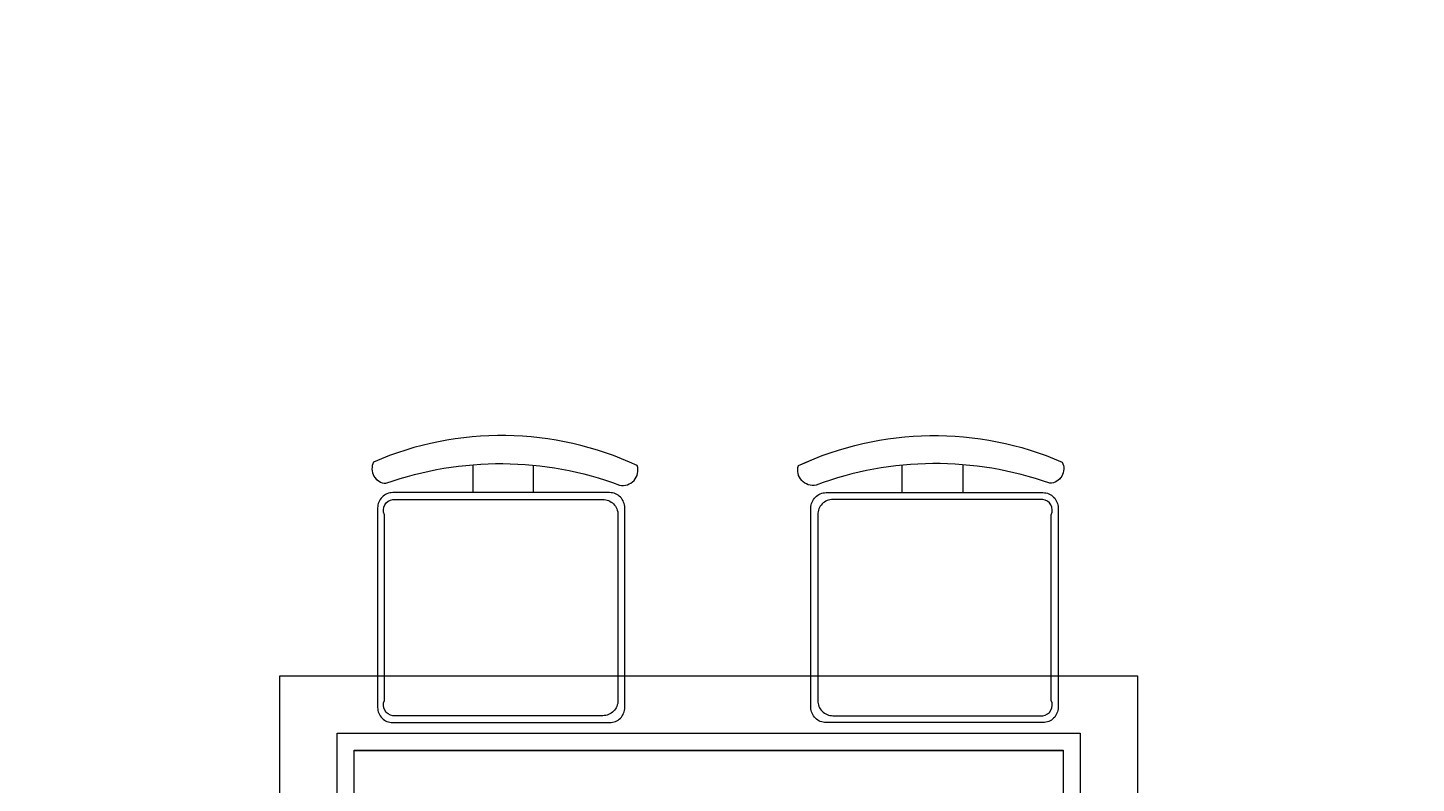
# Model space of a CAD drawing. Units: inches. Extents: x 1962 to 2771, y 1245 to 2660.
# Tile 88 of 114: x 2272 to 2308, y 2284 to 2304. Entities that reach past the tile are written whole.
import ezdxf

# ---------------------------------------------------------------- set-up
doc = ezdxf.new("R2010")
doc.units = ezdxf.units.IN
doc.layers.add('A-ANNO-DIMS', color=2, linetype='Continuous', lineweight=18)
doc.layers.add('A-FURN', color=8, linetype='Continuous', lineweight=13)
doc.styles.get("Standard").update_dxf_attribs({"font": 'arial.ttf'})
doc.dimstyles.get("Standard").update_dxf_attribs({"dimtxt": 0.18, "dimasz": 0.18, "dimexe": 0.18, "dimexo": 0.0625, "dimgap": 0.09, "dimtad": 0, "dimtih": 1, "dimtoh": 1, "dimdec": 4, "dimzin": 0, "dimdsep": 46, "dimtxsty": 'Standard', "dimcen": 0.09, "dimadec": 0, "dimazin": 0, "dimtfac": 1, "dimtdec": 4, "dimtofl": 0, "dimtmove": 0, "dimatfit": 3, "dimfxl": 1, "dimtolj": 1, "dimtzin": 0, "dimarcsym": 0})

# ---------------------------------------------------------------- blocks, each defined once
blk = doc.blocks.new('DINING-TABLE')
for points in [[(0, 13.512), (22.52, 13.512), (22.52, 0), (0, 0)], [(0, 13.512), (22.52, 13.512), (22.52, 0), (0, 0)], [(1.501, 12.011), (21.019, 12.011), (21.019, 1.502), (1.501, 1.502)], [(1.501, 12.011), (21.019, 12.011), (21.019, 1.501), (1.501, 1.501)], [(1.952, 11.561), (20.568, 11.561), (20.568, 1.952), (1.952, 1.952)], [(1.952, 11.56), (20.568, 11.56), (20.568, 1.952), (1.952, 1.952)]]:
    blk.add_lwpolyline(points, close=True)
blk = doc.blocks.new('*D40')
at = {"layer": 'A-ANNO-DIMS', "color": 0, "lineweight": -2, "transparency": 16777216}
for p, q in [((2072.02, 2033.906), (2072.02, 2583.474)), ((2660.807, 2524.406), (2660.807, 2583.474)), ((2072.2, 2583.294), (2366.02, 2583.294)), ((2660.627, 2583.294), (2366.808, 2583.294))]:
    blk.add_line(p, q, dxfattribs=at)
at = {"layer": 'A-ANNO-DIMS', "color": 0, "transparency": 16777216}
for points in [[(2072.2, 2583.324), (2072.2, 2583.264), (2072.02, 2583.294)], [(2660.627, 2583.324), (2660.627, 2583.264), (2660.807, 2583.294)]]:
    blk.add_solid(points, dxfattribs=at)
at = {"layer": 'Defpoints', "color": 0, "transparency": 16777216}
for p in [(2660.807, 2583.294), (2660.807, 2524.344), (2072.02, 2033.844)]:
    blk.add_point(p, dxfattribs=at)
at = {"layer": 'A-ANNO-DIMS', "color": 0, "transparency": 16777216, "insert": (2366.414, 2583.294), "char_height": 0.18, "attachment_point": 5}
blk.add_mtext('\\A1;588.8', dxfattribs=at)

msp = doc.modelspace()

# ---------------------------------------------------------------- linework, layer by layer
at = {"layer": 'A-FURN'}
for points in [[(2281.4134, 2292.1069, -0.1758092), (2287.5472, 2292.0604, 0.5783921), (2288.0119, 2292.5714, 0.2145244), (2281.0881, 2292.6643, 0.552014), (2281.4134, 2292.1069, -0.065079)], [(2281.4134, 2292.1066, -0.1758092), (2287.5472, 2292.0602, 0.5783921), (2288.0119, 2292.5711, 0.2145244), (2281.0881, 2292.6641, 0.552014), (2281.4134, 2292.1066, -0.065079)], [(2292.7111, 2292.0604, -0.5783921), (2292.2464, 2292.5714, -0.2145244), (2299.1703, 2292.6643, -0.552014), (2298.845, 2292.1069, 0.1758092), (2292.7111, 2292.0604)], [(2292.7111, 2292.0602, -0.5783921), (2292.2465, 2292.5711, -0.2145244), (2299.1703, 2292.6641, -0.552014), (2298.845, 2292.1066, 0.1758092), (2292.7112, 2292.0602)], [(2285.2868, 2291.8607), (2285.2868, 2292.5809, -0.0647586)], [(2285.2868, 2291.8605), (2285.2868, 2292.5806, -0.0647586)], [(2294.9716, 2291.8607), (2294.9716, 2292.5809, 0.0647586)], [(2294.9716, 2291.8605), (2294.9716, 2292.5806, 0.0647586)], [(2287.287, 2291.8607), (2281.5925, 2291.8607, 0.4142136), (2281.1941, 2291.4623), (2281.1941, 2286.2263, 0.4142136), (2281.5925, 2285.828), (2287.287, 2285.828, 0.4142136), (2287.6854, 2286.2263), (2287.6854, 2291.4623, 0.4142136), (2287.287, 2291.8607)], [(2287.287, 2291.8605), (2281.5925, 2291.8605, 0.4142136), (2281.1941, 2291.4621), (2281.1941, 2286.2261, 0.4142136), (2281.5925, 2285.8277), (2287.287, 2285.8277, 0.4142136), (2287.6854, 2286.2261), (2287.6854, 2291.4621, 0.4142136), (2287.287, 2291.8605)], [(2298.6658, 2291.8607, -0.4142136), (2299.0642, 2291.4623), (2299.0642, 2286.2263, -0.4142136), (2298.6658, 2285.828), (2292.9714, 2285.828, -0.4142136), (2292.573, 2286.2263), (2292.573, 2291.4623, -0.4142136), (2292.9714, 2291.8607), (2298.6658, 2291.8607)], [(2298.6659, 2291.8605, -0.4142136), (2299.0642, 2291.4621), (2299.0642, 2286.2261, -0.4142136), (2298.6659, 2285.8277), (2292.9714, 2285.8277, -0.4142136), (2292.573, 2286.2261), (2292.573, 2291.4621, -0.4142136), (2292.9714, 2291.8605), (2298.6659, 2291.8605)]]:
    msp.add_lwpolyline(points, format="xyb", dxfattribs=at)
for points in [[(2283.6928, 2292.594), (2283.6928, 2291.8607)], [(2283.6928, 2292.5937), (2283.6928, 2291.8605)], [(2296.5655, 2292.594), (2296.5655, 2291.8607)], [(2296.5655, 2292.5937), (2296.5655, 2291.8605)]]:
    msp.add_lwpolyline(points, dxfattribs=at)
for points in [[(2281.5949, 2291.6812), (2287.1075, 2291.6812, -0.4142136), (2287.5059, 2291.2828), (2287.5059, 2286.4058, -0.4142136), (2287.1075, 2286.0074), (2281.5949, 2286.0074, -0.5120695), (2281.3736, 2286.4058), (2281.3736, 2291.2828, -0.5120695)], [(2281.5949, 2291.681), (2287.1075, 2291.681, -0.4142136), (2287.5059, 2291.2826), (2287.5059, 2286.4056, -0.4142136), (2287.1075, 2286.0072), (2281.5949, 2286.0072, -0.5120695), (2281.3736, 2286.4056), (2281.3736, 2291.2826, -0.5120695)], [(2298.6634, 2291.6812), (2293.1508, 2291.6812, 0.4142136), (2292.7525, 2291.2828), (2292.7525, 2286.4058, 0.4142136), (2293.1508, 2286.0074), (2298.6634, 2286.0074, 0.5120695), (2298.8848, 2286.4058), (2298.8848, 2291.2828, 0.5120695)], [(2298.6634, 2291.681), (2293.1509, 2291.681, 0.4142136), (2292.7525, 2291.2826), (2292.7525, 2286.4056, 0.4142136), (2293.1509, 2286.0072), (2298.6634, 2286.0072, 0.5120695), (2298.8848, 2286.4056), (2298.8848, 2291.2826, 0.5120695)]]:
    msp.add_lwpolyline(points, format="xyb", close=True, dxfattribs=at)

# ---------------------------------------------------------------- block references
msp.add_blockref('DINING-TABLE', (2278.6278, 2273.5392), dxfattribs=at)

# ---------------------------------------------------------------- dimensions: what is measured, and where the dimension line sits
at = {"layer": 'A-ANNO-DIMS'}
dim = msp.add_linear_dim(base=(2660.8074, 2583.2937), p1=(2072.0204, 2033.8437), p2=(2660.8074, 2524.3437), dimstyle='Standard', override={"dimdec": 1, "dimlfac": 1, "dimrnd": 0, "dimzin": 0, "dimdsep": 46, "dimlunit": 2}, dxfattribs=at)
dim.commit()
dim.dimension.update_dxf_attribs({"geometry": '*D40', "text_midpoint": (2366.4139, 2583.2937)})

doc.saveas('drawing.dxf')
